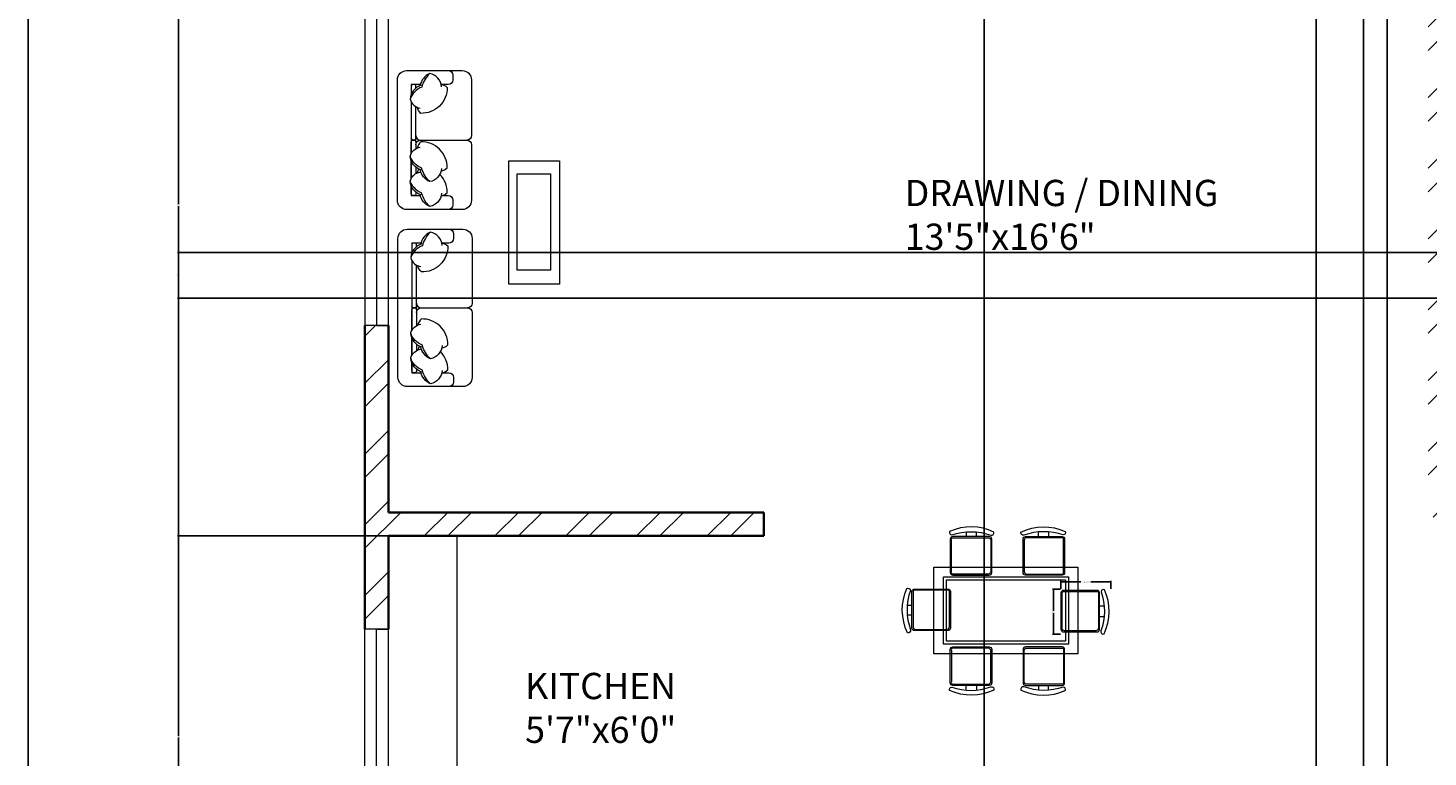
# Model space of a CAD drawing. Units: inches. Extents: x 2064 to 2782, y 1196 to 2299.
# Tile 5 of 11: x 2064 to 2331, y 1963 to 2102. Entities that reach past the tile are written whole.
import ezdxf

# ---------------------------------------------------------------- set-up
doc = ezdxf.new("R2010")
doc.units = ezdxf.units.IN
for name, color, linetype, lineweight in [('A-ANNO-DIMS', 2, 'Continuous', 18), ('A-ANNO-TTLB', 7, 'Continuous', 25), ('A-AREA-IDEN', 7, 'Continuous', 18), ('A-FLOR-CASE', 8, 'Continuous', 18), ('A-FURN', 8, 'Continuous', 13), ('A-GLAZ', 151, 'Continuous', 18), ('A-WALL', 7, 'Continuous', 35), ('A-WALL-PATT', 9, 'Continuous', 13)]:
    doc.layers.add(name, color=color, linetype=linetype, lineweight=lineweight)
doc.styles.get("Standard").update_dxf_attribs({"font": 'arial.ttf'})
doc.dimstyles.get("Standard").update_dxf_attribs({"dimtxt": 0.18, "dimasz": 0.18, "dimexe": 0.18, "dimexo": 0.0625, "dimgap": 0.09, "dimtad": 0, "dimtih": 1, "dimtoh": 1, "dimdec": 4, "dimzin": 0, "dimdsep": 46, "dimtxsty": 'Standard', "dimcen": 0.09, "dimadec": 0, "dimazin": 0, "dimtfac": 1, "dimtdec": 4, "dimtofl": 0, "dimtmove": 0, "dimatfit": 3, "dimfxl": 1, "dimtolj": 1, "dimtzin": 0, "dimarcsym": 0})

# ---------------------------------------------------------------- blocks, each defined once
blk = doc.blocks.new('WIN-60IN')
for p, q in [((0, 4.5), (0, 0)), ((60, 4.5), (0, 4.5)), ((60, 2.25), (60, 4.5)), ((60, 4.5), (60, 0)), ((0, 0), (0, 2.25)), ((0, 2.25), (60, 2.25)), ((0, 0), (60, 0))]:
    blk.add_line(p, q)
blk = doc.blocks.new('WIN-36IN')
for p, q in [((0, 36), (4.5, 36)), ((0, 36), (0, 0)), ((4.5, 36), (2.25, 36)), ((2.25, 36), (2.25, 0)), ((4.5, 36), (4.5, 0)), ((2.25, 0), (0, 0)), ((0, 0), (4.5, 0))]:
    blk.add_line(p, q)
blk = doc.blocks.new('CHAIR-DINING')
for points in [[(7.35, 7.85, 0.414214), (6.87, 8.33), (0.49, 8.33, 0.414214), (0, 7.85), (0, 0.91, 0.414214), (0.49, 0.42), (6.87, 0.42, 0.414214), (7.35, 0.91), (7.35, 7.85)], [(7.35, 7.85, 0.414214), (6.87, 8.33), (0.49, 8.33, 0.414214), (0, 7.85), (0, 0.91, 0.414214), (0.49, 0.42), (6.87, 0.42, 0.414214), (7.35, 0.91), (7.35, 7.85)], [(7.65, 8.06, -0.175809), (7.6, 0.59, 0.578392), (8.22, 0.02, 0.214524), (8.33, 8.46, 0.552014), (7.65, 8.06, -0.065079)], [(7.65, 8.06, -0.175809), (7.6, 0.59, 0.578392), (8.22, 0.02, 0.214524), (8.33, 8.46, 0.552014), (7.65, 8.06, -0.065079)], [(7.35, 3.34), (8.23, 3.34, -0.064759)], [(7.35, 3.34), (8.23, 3.34, -0.064759)]]:
    blk.add_lwpolyline(points, format="xyb")
for points in [[(7.13, 7.84), (7.13, 1.13, -0.414214), (6.65, 0.64), (0.7, 0.64, -0.414214), (0.22, 1.13), (0.22, 7.84, -0.512069), (0.7, 8.11), (6.65, 8.11, -0.512069)], [(7.13, 7.84), (7.13, 1.12, -0.414214), (6.65, 0.64), (0.7, 0.64, -0.414214), (0.22, 1.12), (0.22, 7.84, -0.512069), (0.7, 8.11), (6.65, 8.11, -0.512069)]]:
    blk.add_lwpolyline(points, format="xyb", close=True)
blk.add_lwpolyline([(8.25, 5.29), (7.35, 5.29)])
blk.add_lwpolyline([(8.25, 5.29), (7.35, 5.29)])
blk = doc.blocks.new('TABLE-DINING')
for points in [[(0, 16.47), (27.45, 16.47), (27.45, 0), (0, 0)], [(0, 16.47), (27.45, 16.47), (27.45, 0), (0, 0)], [(1.83, 14.64), (25.62, 14.64), (25.62, 1.83), (1.83, 1.83)], [(1.83, 14.64), (25.62, 14.64), (25.62, 1.83), (1.83, 1.83)], [(2.38, 14.09), (25.07, 14.09), (25.07, 2.38), (2.38, 2.38)], [(2.38, 14.09), (25.07, 14.09), (25.07, 2.38), (2.38, 2.38)]]:
    blk.add_lwpolyline(points, close=True)
blk = doc.blocks.new('TABLE-COFFEE')
for points in [[(0, 23.5), (9.66, 23.5), (9.66, 0), (0, 0)], [(1.54, 21.03), (7.9, 21.03), (7.9, 2.7), (1.54, 2.7)]]:
    blk.add_lwpolyline(points, close=True)
blk = doc.blocks.new('*D18')
at = {"layer": 'A-ANNO-DIMS', "color": 0, "lineweight": -2, "transparency": 16777216}
for p, q in [((2260.79, 1994.7), (2260.79, 1996.25)), ((2260.97, 1996.07), (2264.58, 1996.07)), ((2270.11, 1996.07), (2266.49, 1996.07)), ((2270.29, 1994.7), (2270.29, 1996.25))]:
    blk.add_line(p, q, dxfattribs=at)
at = {"layer": 'A-ANNO-DIMS', "color": 0, "transparency": 16777216}
for points in [[(2260.97, 1996.1), (2260.97, 1996.04), (2260.79, 1996.07)], [(2270.11, 1996.1), (2270.11, 1996.04), (2270.29, 1996.07)]]:
    blk.add_solid(points, dxfattribs=at)
at = {"layer": 'Defpoints', "color": 0, "transparency": 16777216}
for p in [(2270.29, 1996.07), (2260.79, 1994.64), (2270.29, 1994.64)]:
    blk.add_point(p, dxfattribs=at)
at = {"layer": 'A-ANNO-DIMS', "color": 0, "transparency": 16777216, "insert": (2265.54, 1996.07), "char_height": 0.18, "attachment_point": 5}
blk.add_mtext('\\A1;CHAIR 10 TYP.', dxfattribs=at)
blk = doc.blocks.new('*D19')
at = {"layer": 'A-ANNO-DIMS', "color": 0, "lineweight": -2, "transparency": 16777216}
for p, q in [((2260.72, 1994.64), (2259.18, 1994.64)), ((2259.36, 1994.46), (2259.36, 1990.54)), ((2259.36, 1986.26), (2259.36, 1990.18)), ((2260.72, 1986.08), (2259.18, 1986.08))]:
    blk.add_line(p, q, dxfattribs=at)
at = {"layer": 'A-ANNO-DIMS', "color": 0, "transparency": 16777216}
for points in [[(2259.33, 1994.46), (2259.39, 1994.46), (2259.36, 1994.64)], [(2259.33, 1986.26), (2259.39, 1986.26), (2259.36, 1986.08)]]:
    blk.add_solid(points, dxfattribs=at)
at = {"layer": 'Defpoints', "color": 0, "transparency": 16777216}
for p in [(2259.36, 1994.64), (2260.79, 1994.64), (2260.79, 1986.08)]:
    blk.add_point(p, dxfattribs=at)
at = {"layer": 'A-ANNO-DIMS', "color": 0, "transparency": 16777216, "insert": (2259.36, 1990.36), "char_height": 0.18, "attachment_point": 5}
blk.add_mtext('\\A1;9 TYP.', dxfattribs=at)
blk = doc.blocks.new('*D26')
at = {"layer": 'A-ANNO-DIMS', "color": 0, "lineweight": -2, "transparency": 16777216}
for p, q in [((2246.18, 1643.35), (2246.18, 2269.97)), ((2246.36, 2269.79), (2281.92, 2269.79)), ((2318.27, 2269.79), (2282.71, 2269.79)), ((2318.45, 1640.85), (2318.45, 2269.97))]:
    blk.add_line(p, q, dxfattribs=at)
at = {"layer": 'A-ANNO-DIMS', "color": 0, "transparency": 16777216}
for points in [[(2246.36, 2269.82), (2246.36, 2269.76), (2246.18, 2269.79)], [(2318.27, 2269.82), (2318.27, 2269.76), (2318.45, 2269.79)]]:
    blk.add_solid(points, dxfattribs=at)
at = {"layer": 'Defpoints', "color": 0, "transparency": 16777216}
for p in [(2318.45, 2269.79), (2246.18, 1643.29), (2318.45, 1640.79)]:
    blk.add_point(p, dxfattribs=at)
at = {"layer": 'A-ANNO-DIMS', "color": 0, "transparency": 16777216, "insert": (2282.32, 2269.79), "char_height": 0.18, "attachment_point": 5}
blk.add_mtext('\\A1;72.27', dxfattribs=at)
blk = doc.blocks.new('*D31')
at = {"layer": 'A-ANNO-DIMS', "color": 0, "lineweight": -2, "transparency": 16777216}
for p, q in [((2132.61, 2004.79), (2092.49, 2004.79)), ((2092.67, 2004.61), (2092.67, 1966.72)), ((2092.67, 1928.47), (2092.67, 1966.36)), ((2132.61, 1928.29), (2092.49, 1928.29))]:
    blk.add_line(p, q, dxfattribs=at)
at = {"layer": 'A-ANNO-DIMS', "color": 0, "transparency": 16777216}
for points in [[(2092.64, 2004.61), (2092.7, 2004.61), (2092.67, 2004.79)], [(2092.64, 1928.47), (2092.7, 1928.47), (2092.67, 1928.29)]]:
    blk.add_solid(points, dxfattribs=at)
at = {"layer": 'Defpoints', "color": 0, "transparency": 16777216}
for p in [(2092.67, 2004.79), (2132.67, 2004.79), (2132.67, 1928.29)]:
    blk.add_point(p, dxfattribs=at)
at = {"layer": 'A-ANNO-DIMS', "color": 0, "transparency": 16777216, "insert": (2092.67, 1966.54), "char_height": 0.18, "attachment_point": 5}
blk.add_mtext('\\A1;76.5', dxfattribs=at)
blk = doc.blocks.new('*D32')
at = {"layer": 'A-ANNO-DIMS', "color": 0, "lineweight": -2, "transparency": 16777216}
for p, q in [((2132.61, 2130.79), (2092.49, 2130.79)), ((2092.67, 2130.61), (2092.67, 2067.97)), ((2092.67, 2004.97), (2092.67, 2067.61)), ((2132.61, 2004.79), (2092.49, 2004.79))]:
    blk.add_line(p, q, dxfattribs=at)
at = {"layer": 'A-ANNO-DIMS', "color": 0, "transparency": 16777216}
for points in [[(2092.64, 2130.61), (2092.7, 2130.61), (2092.67, 2130.79)], [(2092.64, 2004.97), (2092.7, 2004.97), (2092.67, 2004.79)]]:
    blk.add_solid(points, dxfattribs=at)
at = {"layer": 'Defpoints', "color": 0, "transparency": 16777216}
for p in [(2092.67, 2130.79), (2132.67, 2130.79), (2132.67, 2004.79)]:
    blk.add_point(p, dxfattribs=at)
at = {"layer": 'A-ANNO-DIMS', "color": 0, "transparency": 16777216, "insert": (2092.67, 2067.79), "char_height": 0.18, "attachment_point": 5}
blk.add_mtext('\\A1;126', dxfattribs=at)
blk = doc.blocks.new('*D35')
at = {"layer": 'A-ANNO-DIMS', "color": 0, "lineweight": -2, "transparency": 16777216}
for p, q in [((2309.4, 1932.85), (2309.4, 2269.97)), ((2309.58, 2269.79), (2347.37, 2269.79)), ((2385.94, 2269.79), (2348.16, 2269.79)), ((2386.12, 1856.35), (2386.12, 2269.97))]:
    blk.add_line(p, q, dxfattribs=at)
at = {"layer": 'A-ANNO-DIMS', "color": 0, "transparency": 16777216}
for points in [[(2309.58, 2269.82), (2309.58, 2269.76), (2309.4, 2269.79)], [(2385.94, 2269.82), (2385.94, 2269.76), (2386.12, 2269.79)]]:
    blk.add_solid(points, dxfattribs=at)
at = {"layer": 'Defpoints', "color": 0, "transparency": 16777216}
for p in [(2386.12, 2269.79), (2309.4, 1932.79), (2386.12, 1856.29)]:
    blk.add_point(p, dxfattribs=at)
at = {"layer": 'A-ANNO-DIMS', "color": 0, "transparency": 16777216, "insert": (2347.76, 2269.79), "char_height": 0.18, "attachment_point": 5}
blk.add_mtext('\\A1;76.72', dxfattribs=at)
blk = doc.blocks.new('*D39')
at = {"layer": 'A-ANNO-DIMS', "color": 0, "lineweight": -2, "transparency": 16777216}
for p, q in [((2322.95, 1645.35), (2322.95, 2269.97)), ((2323.13, 2269.79), (2333.59, 2269.79)), ((2344.97, 2269.79), (2334.51, 2269.79)), ((2345.15, 1645.35), (2345.15, 2269.97))]:
    blk.add_line(p, q, dxfattribs=at)
at = {"layer": 'A-ANNO-DIMS', "color": 0, "transparency": 16777216}
for points in [[(2323.13, 2269.82), (2323.13, 2269.76), (2322.95, 2269.79)], [(2344.97, 2269.82), (2344.97, 2269.76), (2345.15, 2269.79)]]:
    blk.add_solid(points, dxfattribs=at)
at = {"layer": 'Defpoints', "color": 0, "transparency": 16777216}
for p in [(2345.15, 2269.79), (2322.95, 1645.29), (2345.15, 1645.29)]:
    blk.add_point(p, dxfattribs=at)
at = {"layer": 'A-ANNO-DIMS', "color": 0, "transparency": 16777216, "insert": (2334.05, 2269.79), "char_height": 0.18, "attachment_point": 5}
blk.add_mtext('\\A1;22.194', dxfattribs=at)
blk = doc.blocks.new('*D40')
at = {"layer": 'A-ANNO-DIMS', "color": 0, "lineweight": -2, "transparency": 16777216}
for p, q in [((2648.61, 2058.79), (2092.49, 2058.79)), ((2092.67, 2058.61), (2092.67, 2054.63)), ((2092.67, 2050.29), (2092.67, 2054.27)), ((2648.61, 2050.11), (2092.49, 2050.11))]:
    blk.add_line(p, q, dxfattribs=at)
at = {"layer": 'A-ANNO-DIMS', "color": 0, "transparency": 16777216}
for points in [[(2092.64, 2058.61), (2092.7, 2058.61), (2092.67, 2058.79)], [(2092.64, 2050.29), (2092.7, 2050.29), (2092.67, 2050.11)]]:
    blk.add_solid(points, dxfattribs=at)
at = {"layer": 'Defpoints', "color": 0, "transparency": 16777216}
for p in [(2092.67, 2058.79), (2648.67, 2058.79), (2648.67, 2050.11)]:
    blk.add_point(p, dxfattribs=at)
at = {"layer": 'A-ANNO-DIMS', "color": 0, "transparency": 16777216, "insert": (2092.67, 2054.45), "char_height": 0.18, "attachment_point": 5}
blk.add_mtext('\\A1;8.682', dxfattribs=at)

msp = doc.modelspace()

# ---------------------------------------------------------------- hatches: boundary and pattern name
at = {"layer": 'A-WALL-PATT'}
h = msp.add_hatch(dxfattribs=at)
h.set_pattern_fill('ANSI32', color=256)
h.paths.add_polyline_path([(2489.7688, 2189.2917), (2574.5454, 2189.2917), (2574.5454, 2191.5417), (2574.5454, 2193.7917), (2570.6691, 2193.7917), (2570.6691, 2197.3052), (2568.4191, 2197.3052), (2566.1691, 2197.3052), (2566.1691, 2193.7917), (2494.1691, 2193.7917), (2494.1691, 2229.7917), (2523.2441, 2229.7917), (2523.2441, 2234.2917), (2471.2886, 2234.2917), (2471.2886, 2229.7917), (2489.6691, 2229.7917), (2489.6691, 2193.7917), (2417.6691, 2193.7917), (2417.6691, 2197.0632), (2415.4191, 2197.0632), (2413.1691, 2197.0632), (2413.1691, 2193.7917), (2406.8865, 2193.7917), (2406.8865, 2189.2917), (2485.2688, 2189.2917), (2485.2688, 2063.2917), (2369.1629, 2063.2917), (2369.1629, 2058.7917), (2386.1222, 2058.7917), (2386.1222, 1856.2917), (2382.1576, 1856.2917), (2382.1576, 1851.7917), (2394.9764, 1851.7917), (2394.9764, 1854.0417), (2394.9764, 1856.2917), (2390.6222, 1856.2917), (2390.6222, 2058.7917), (2485.2688, 2058.7917), (2493.762, 2058.7917), (2493.762, 2061.0417), (2493.762, 2063.2917), (2489.7688, 2063.2917)])
h.paths.add_polyline_path([(2447.2886, 2234.2917), (2413.1691, 2234.2917), (2413.1691, 2217.3799), (2417.6691, 2217.3799), (2417.6691, 2229.7917), (2447.2886, 2229.7917)], flags=17)
h.paths.add_polyline_path([(2570.6691, 2234.2917), (2547.2441, 2234.2917), (2547.2441, 2229.7917), (2566.1691, 2229.7917), (2566.1691, 2216.5615), (2570.6691, 2216.5615)], flags=17)
h.paths.add_polyline_path([(2653.1691, 2189.2917), (2653.1691, 2193.7917), (2640.8843, 2193.7917), (2640.8843, 2189.2917), (2648.6691, 2189.2917), (2648.6691, 2162.7138), (2653.1691, 2162.7138)])
h.paths.add_polyline_path([(2653.1691, 2102.7138), (2648.6691, 2102.7138), (2648.6691, 2063.2917), (2526.7281, 2063.2917), (2526.7281, 2058.7917), (2541.1691, 2058.7917), (2541.1691, 1993.2917), (2545.6691, 1993.2917), (2545.6691, 1997.7917), (2545.6691, 2058.7917), (2648.6691, 2058.7917), (2648.6691, 2050.1099), (2653.1691, 2050.1099)])
h.paths.add_polyline_path([(2600.6691, 1856.2917), (2493.4607, 1856.2917), (2493.4607, 1851.7917), (2596.1691, 1851.7917), (2596.1691, 1695.7917), (2594.0816, 1695.7917), (2594.0816, 1691.2917), (2614.7905, 1691.2917), (2614.7905, 1645.2917), (2536.7905, 1645.2917), (2536.7905, 1691.2917), (2539.332, 1691.2917), (2539.332, 1693.5417), (2539.332, 1695.7917), (2452.1691, 1695.7917), (2452.1691, 1851.7917), (2456.0775, 1851.7917), (2456.0775, 1856.2917), (2427.1536, 1856.2917), (2427.1536, 1851.7917), (2447.6691, 1851.7917), (2447.6691, 1695.7917), (2447.6691, 1645.2917), (2405.1469, 1645.2917), (2405.1469, 1640.7917), (2452.1691, 1640.7917), (2452.1691, 1645.2917), (2452.1691, 1691.2917), (2534.7905, 1691.2917), (2534.7905, 1645.2917), (2534.7905, 1643.2917), (2614.7905, 1643.2917), (2616.7905, 1643.2917), (2616.7905, 1691.2917), (2622.4029, 1691.2917), (2622.4029, 1693.7143), (2622.4029, 1695.7917), (2600.6691, 1695.7917), (2600.6691, 1779.7917), (2648.6691, 1779.7917), (2648.6691, 1695.7917), (2646.4029, 1695.7917), (2646.4029, 1691.2917), (2653.1691, 1691.2917), (2653.1691, 1906.3508), (2648.6691, 1906.3508), (2648.6691, 1856.2917), (2648.6691, 1784.2917), (2600.6691, 1784.2917)])
h.paths.add_polyline_path([(2322.9532, 1819.5181), (2320.7032, 1819.5181), (2318.4532, 1819.5181), (2318.4532, 1695.7917), (2242.7664, 1695.7917), (2242.7664, 1691.2917), (2318.4532, 1691.2917), (2318.4532, 1640.7917), (2322.9532, 1640.7917), (2345.1469, 1640.7917), (2345.1469, 1643.0417), (2345.1469, 1645.2917), (2322.9532, 1645.2917), (2322.9532, 1691.2917), (2322.9532, 1695.7917)])
h.paths.add_polyline_path([(2166.1825, 1691.2917), (2164.1825, 1691.2917), (2164.1825, 1643.2917), (2166.1825, 1643.2917), (2246.1825, 1643.2917), (2246.1825, 1645.2917), (2246.1825, 1691.2917), (2244.1825, 1691.2917), (2244.1825, 1645.2917), (2166.1825, 1645.2917)])
h.paths.add_polyline_path([(2309.404, 1932.7917), (2204.1691, 1932.7917), (2204.1691, 1960.0962), (2199.6691, 1960.0962), (2199.6691, 1932.7917), (2132.6691, 1932.7917), (2132.6691, 1951.0737), (2128.1691, 1951.0737), (2128.1691, 1910.0412), (2132.6691, 1910.0412), (2132.6691, 1928.2917), (2304.904, 1928.2917), (2304.904, 1856.2917), (2304.904, 1851.7917), (2318.4532, 1851.7917), (2318.4532, 1848.8308), (2322.9532, 1848.8308), (2322.9532, 1851.7917), (2347.7631, 1851.7917), (2347.7631, 1856.2917), (2309.404, 1856.2917)])
h.paths.add_polyline_path([(2132.6691, 2044.9092), (2130.4191, 2044.9092), (2128.1691, 2044.9092), (2128.1691, 1987.0737), (2132.6691, 1987.0737), (2132.6691, 2004.7917), (2199.6691, 2004.7917), (2204.1691, 2004.7917), (2204.1691, 2009.2917), (2132.6691, 2009.2917)])
h.paths.add_polyline_path([(2186.6691, 2195.9329), (2184.4191, 2195.9329), (2184.4191, 2195.8929), (2182.1691, 2195.9329), (2182.1691, 2193.7917), (2128.1691, 2193.7917), (2128.1691, 2181.4967), (2132.6691, 2181.4967), (2132.6691, 2182.7769), (2132.6691, 2189.2917), (2182.1691, 2189.2917), (2182.1691, 2135.2917), (2179.804, 2135.2917), (2179.804, 2130.7917), (2190.215, 2130.7917), (2190.215, 2133.0417), (2190.215, 2135.2917), (2186.6691, 2135.2917)])
h.paths.add_polyline_path([(2340.0628, 2189.2917), (2340.0628, 2191.5417), (2340.0628, 2193.7917), (2335.1691, 2193.7917), (2335.1691, 2234.2917), (2280.6746, 2234.2917), (2280.6746, 2229.7917), (2330.6691, 2229.7917), (2330.6691, 2193.7917), (2330.6691, 2135.2917), (2218.6309, 2135.2917), (2218.6309, 2130.7917), (2330.7688, 2130.7917), (2330.7688, 2008.4023), (2335.2688, 2008.4023), (2335.2688, 2058.7917), (2338.9208, 2058.7917), (2338.9208, 2061.0417), (2338.9208, 2063.2917), (2335.2688, 2063.2917), (2335.2688, 2189.2917)])
h.paths.add_polyline_path([(2220.6746, 2234.2917), (2182.1691, 2234.2917), (2182.1691, 2227.4187), (2186.6691, 2227.4187), (2186.6691, 2229.7917), (2220.6746, 2229.7917), (2220.6746, 2232.0417)])
h.paths.add_polyline_path([(2158.8146, 2135.2917), (2132.6691, 2135.2917), (2132.6691, 2157.4967), (2128.1691, 2157.4967), (2128.1691, 2104.9092), (2132.6691, 2104.9092), (2132.6691, 2130.7917), (2158.8146, 2130.7917), (2158.8146, 2133.0417)])
h.paths.add_polyline_path([(2396.0464, 2062.2045), (2434.8868, 2062.2045), (2434.8868, 2080.8619), (2396.0464, 2080.8619)], flags=24)
h.paths.add_polyline_path([(2196.1396, 1653.3449), (2232.023, 1653.3449), (2232.023, 1672.0022), (2196.1396, 1672.0022)], flags=25)

# ---------------------------------------------------------------- linework, layer by layer
at = {"layer": 'A-ANNO-TTLB'}
msp.add_lwpolyline([(2063.9994, 2298.574), (2782.0941, 2298.574), (2782.0941, 1490.6238), (2063.9994, 1490.6238)], close=True, dxfattribs=at)
at = {"layer": 'A-FLOR-CASE'}
msp.add_line((2145.6809, 2004.7917), (2145.6809, 1946.3811), dxfattribs=at)
at = {"layer": 'A-FURN', "ltscale": 0.03}
for points in [[(2148.4815, 2081.0868, -0.41421356), (2147.5995, 2080.2048, -0.41421356), (2148.4815, 2079.3228), (2148.4815, 2068.7388, -0.41421356), (2146.7175, 2066.9749), (2136.1335, 2066.9749, -0.41421356), (2134.3695, 2068.7388), (2134.3695, 2091.6708, -0.41421356), (2136.1335, 2093.4348), (2146.7175, 2093.4348, -0.41421356), (2148.4815, 2091.6708), (2148.4815, 2081.0868, -0.41421356), (2147.5995, 2080.2048, -0.41421356), (2148.4815, 2079.3228)], [(2148.6, 2049.114, -0.41421356), (2147.718, 2048.232, -0.41421356), (2148.6, 2047.35), (2148.6, 2035.002, -0.41421356), (2146.836, 2033.238), (2136.252, 2033.238, -0.41421356), (2134.488, 2035.002), (2134.488, 2061.4619, -0.41421356), (2136.252, 2063.2259), (2146.836, 2063.2259, -0.41421356), (2148.6, 2061.4619), (2148.6, 2049.114, -0.41421356), (2147.718, 2048.232, -0.41421356), (2148.6, 2047.35)]]:
    msp.add_lwpolyline(points, format="xyb", dxfattribs=at)
at = {"layer": 'A-FURN'}
for points in [[(2140.5352, 2092.8734, 0.14772988), (2139.0194, 2090.2956, 0.21334276), (2136.7962, 2088.0211, 0.17866181)], [(2142.7584, 2090.3462, 0.35677236), (2140.5352, 2092.8734, 0.24954205), (2138.7031, 2090.5835, -9.61688035)], [(2144.0715, 2093.4348, -0.41421356), (2144.9535, 2092.5528), (2144.9535, 2091.6708, -0.41421356), (2144.0715, 2090.7888), (2142.705, 2090.7888)], [(2138.8986, 2090.6517, 0.30666349), (2136.7962, 2088.0211, 0.30632997), (2138.7162, 2086.3025, -0.87284716)], [(2137.8975, 2090.1157), (2137.8975, 2090.436, 0.41421356), (2137.5447, 2090.7888), (2137.3683, 2090.7888, 0.41421356), (2137.0155, 2090.436)], [(2137.0155, 2090.436), (2137.0155, 2088.9333, 0.41421356)], [(2142.7046, 2090.7907, -0.16554063), (2143.8699, 2090.2451, -0.42598917), (2138.8173, 2085.2916, -0.12152332), (2138.1209, 2086.4675, 7.11546429)], [(2137.0155, 2087.466), (2137.0155, 2080.5576, 0.41421356), (2137.3683, 2080.2048), (2137.5447, 2080.2048, 0.41421356), (2137.8975, 2080.5576), (2137.8975, 2086.5779, 0.41421356)], [(2137.8975, 2081.0868, 0.41421356), (2138.7795, 2080.2048)], [(2137.8975, 2081.0868, 0.41421356), (2138.7795, 2080.2048), (2147.5995, 2080.2048, 0.41421356)], [(2138.8986, 2074.5092, -0.30666349), (2136.7962, 2077.1398, -0.30632997), (2138.7162, 2078.8584, 0.87284716)], [(2137.0155, 2077.6949), (2137.0155, 2079.852, -0.41421356), (2137.3683, 2080.2048), (2137.5447, 2080.2048, -0.41421356), (2137.8975, 2079.852), (2137.8975, 2078.583, -0.41421356)], [(2137.8975, 2079.3228, -0.41421356), (2138.7795, 2080.2048)], [(2137.8975, 2079.3228, -0.41421356), (2138.7795, 2080.2048), (2147.5995, 2080.2048, -0.41421356)], [(2142.7046, 2074.3702, 0.16554063), (2143.8699, 2074.9158, 0.42598917), (2138.8173, 2079.8693, 0.12152332), (2138.1209, 2078.6935, -7.11546429)], [(2140.5352, 2072.2875, -0.14772988), (2139.0194, 2074.8653, -0.21334276), (2136.7962, 2077.1398, -0.17866181)], [(2137.0155, 2072.9436), (2137.0155, 2076.2276, -0.41421356)], [(2138.8986, 2069.7579, -0.30666349), (2136.7962, 2072.3886, -0.30632997), (2138.7162, 2074.1071, 0.87284716)], [(2137.8975, 2075.0452), (2137.8975, 2073.8318, -0.41421356)], [(2138.4657, 2074.6816, 0.07186538), (2138.1209, 2073.9422, -7.11546429)], [(2142.7584, 2074.8148, -0.35677236), (2140.5352, 2072.2875, -0.24954205), (2138.7031, 2074.5774, 9.61688035)], [(2142.7046, 2069.6189, 0.16554063), (2143.8699, 2070.1646, 0.20023115), (2142.4506, 2073.6658, 0.12152332)], [(2140.5352, 2067.5362, -0.14772988), (2139.0194, 2070.114, -0.21334276), (2136.7962, 2072.3886, -0.17866181)], [(2137.0155, 2069.9736), (2137.0155, 2071.4763, -0.41421356)], [(2137.0155, 2071.4763), (2137.0155, 2069.6208), (2138.7489, 2069.6208, -0.41421356)], [(2137.8975, 2070.2939), (2137.8975, 2069.9736, -0.41421356), (2137.5447, 2069.6208), (2137.3683, 2069.6208, -0.41421356), (2137.0155, 2069.9736)], [(2142.7584, 2070.0635, -0.35677236), (2140.5352, 2067.5362, -0.24954205), (2138.7031, 2069.8261, 9.61688035)], [(2142.705, 2069.6208), (2144.0715, 2069.6208, -0.41421356), (2144.9535, 2068.7388), (2144.9535, 2067.8569, -0.41421356), (2144.0715, 2066.9749)], [(2140.6537, 2062.6646, 0.14772988), (2139.1379, 2060.0868, 0.21334276), (2136.9147, 2057.8122, 0.17866181)], [(2142.8769, 2060.1373, 0.35677236), (2140.6537, 2062.6646, 0.24954205), (2138.8216, 2060.3746, -9.61688035)], [(2144.19, 2063.2259, -0.41421356), (2145.072, 2062.3439), (2145.072, 2061.4619, -0.41421356), (2144.19, 2060.5799), (2142.8235, 2060.5799)], [(2139.0171, 2060.4429, 0.30666349), (2136.9147, 2057.8122, 0.30632997), (2138.8347, 2056.0937, -0.87284716)], [(2138.016, 2059.9069), (2138.016, 2060.2271, 0.41421356), (2137.6632, 2060.5799), (2137.4868, 2060.5799, 0.41421356), (2137.134, 2060.2271)], [(2137.134, 2060.2271), (2137.134, 2058.7244, 0.41421356)], [(2142.8231, 2060.5818, -0.16554063), (2143.9884, 2060.0362, -0.42598917), (2138.9358, 2055.0827, -0.12152332), (2138.2393, 2056.2586, 7.11546429)], [(2137.134, 2057.2571), (2137.134, 2048.5848, 0.41421356), (2137.4868, 2048.232), (2137.6632, 2048.232, 0.41421356), (2138.016, 2048.5848), (2138.016, 2056.369, 0.41421356)], [(2138.016, 2049.114, 0.41421356), (2138.898, 2048.232)], [(2138.016, 2049.114, 0.41421356), (2138.898, 2048.232), (2147.718, 2048.232, 0.41421356)], [(2137.134, 2043.9581), (2137.134, 2047.8792, -0.41421356), (2137.4868, 2048.232), (2137.6632, 2048.232, -0.41421356), (2138.016, 2047.8792), (2138.016, 2044.8462, -0.41421356)], [(2138.016, 2047.35, -0.41421356), (2138.898, 2048.232)], [(2138.016, 2047.35, -0.41421356), (2138.898, 2048.232), (2147.718, 2048.232, -0.41421356)], [(2142.8231, 2040.6334, 0.16554063), (2143.9884, 2041.179, 0.42598917), (2138.9358, 2046.1325, 0.12152332), (2138.2393, 2044.9566, -7.11546429)], [(2139.0171, 2040.7723, -0.30666349), (2136.9147, 2043.403, -0.30632997), (2138.8347, 2045.1216, 0.87284716)], [(2140.6537, 2038.5506, -0.14772988), (2139.1379, 2041.1285, -0.21334276), (2136.9147, 2043.403, -0.17866181)], [(2137.134, 2039.2068), (2137.134, 2042.4908, -0.41421356)], [(2138.016, 2041.3084), (2138.016, 2040.0949, -0.41421356)], [(2138.5842, 2040.9448, 0.07186538), (2138.2393, 2040.2053, -7.11546429)], [(2142.8769, 2041.0779, -0.35677236), (2140.6537, 2038.5506, -0.24954205), (2138.8216, 2040.8406, 9.61688035)], [(2139.0171, 2036.021, -0.30666349), (2136.9147, 2038.6517, -0.30632997), (2138.8347, 2040.3703, 0.87284716)], [(2140.6537, 2033.7993, -0.14772988), (2139.1379, 2036.3772, -0.21334276), (2136.9147, 2038.6517, -0.17866181)], [(2137.134, 2037.7395), (2137.134, 2035.884), (2138.8674, 2035.884, -0.41421356)], [(2137.134, 2036.2368), (2137.134, 2037.7395, -0.41421356)], [(2142.8231, 2035.8821, 0.16554063), (2143.9884, 2036.4277, 0.20023115), (2142.5691, 2039.9289, 0.12152332)], [(2138.016, 2036.5571), (2138.016, 2036.2368, -0.41421356), (2137.6632, 2035.884), (2137.4868, 2035.884, -0.41421356), (2137.134, 2036.2368)], [(2142.8769, 2036.3266, -0.35677236), (2140.6537, 2033.7993, -0.24954205), (2138.8216, 2036.0893, 9.61688035)], [(2142.8235, 2035.884), (2144.19, 2035.884, -0.41421356), (2145.072, 2035.002), (2145.072, 2034.12, -0.41421356), (2144.19, 2033.238)], [(2239.9772, 2004.9849, -0.17580919), (2247.4526, 2004.9283, 0.57839206), (2248.019, 2005.551, 0.21452438), (2239.5808, 2005.6643, 0.55201397), (2239.9772, 2004.9849, -0.06507904)], [(2239.9772, 2004.9846, -0.17580919), (2247.4527, 2004.928, 0.57839206), (2248.019, 2005.5508, 0.21452438), (2239.5808, 2005.664, 0.55201397), (2239.9772, 2004.9846, -0.06507904)], [(2253.746, 2004.9283, -0.57839206), (2253.1797, 2005.551, -0.21452438), (2261.6179, 2005.6643, -0.55201397), (2261.2214, 2004.9849, 0.1758092), (2253.746, 2004.9283)], [(2253.746, 2004.928, -0.57839206), (2253.1797, 2005.5508, -0.21452438), (2261.6179, 2005.664, -0.55201397), (2261.2214, 2004.9846, 0.1758092), (2253.746, 2004.928)], [(2247.1355, 2004.6849), (2240.1955, 2004.6849, 0.41421356), (2239.71, 2004.1994), (2239.71, 1997.8182, 0.41421356), (2240.1955, 1997.3327), (2247.1355, 1997.3327, 0.41421356), (2247.621, 1997.8182), (2247.621, 2004.1994, 0.41421356), (2247.1355, 2004.6849)], [(2247.1355, 2004.6846), (2240.1956, 2004.6846, 0.41421356), (2239.71, 2004.1991), (2239.71, 1997.8179, 0.41421356), (2240.1956, 1997.3324), (2247.1355, 1997.3324, 0.41421356), (2247.621, 1997.8179), (2247.621, 2004.1991, 0.41421356), (2247.1355, 2004.6846)], [(2244.6978, 2004.6849), (2244.6978, 2005.5626, -0.06475861)], [(2244.6978, 2004.6846), (2244.6978, 2005.5623, -0.06475861)], [(2261.0031, 2004.6849, -0.41421356), (2261.4886, 2004.1994), (2261.4886, 1997.8182, -0.41421356), (2261.0031, 1997.3327), (2254.0631, 1997.3327, -0.41421356), (2253.5776, 1997.8182), (2253.5776, 2004.1994, -0.41421356), (2254.0631, 2004.6849), (2261.0031, 2004.6849)], [(2261.0031, 2004.6846, -0.41421356), (2261.4886, 2004.1991), (2261.4886, 1997.8179, -0.41421356), (2261.0031, 1997.3324), (2254.0632, 1997.3324, -0.41421356), (2253.5776, 1997.8179), (2253.5776, 2004.1991, -0.41421356), (2254.0632, 2004.6846), (2261.0031, 2004.6846)], [(2256.5008, 2004.6849), (2256.5008, 2005.5626, 0.06475861)], [(2256.5008, 2004.6846), (2256.5008, 2005.5623, 0.06475861)], [(2232.1565, 1986.9329, -0.57839206), (2231.5337, 1986.3666, -0.21452438), (2231.4205, 1994.8048, -0.55201397), (2232.0998, 1994.4083, 0.17580937), (2232.1565, 1986.9329)], [(2232.1565, 1986.9326, -0.57839206), (2231.5338, 1986.3663, -0.21452438), (2231.4205, 1994.8045, -0.55201397), (2232.0999, 1994.408, 0.17580937), (2232.1565, 1986.9326)], [(2232.3999, 1994.19, -0.41421356), (2232.8854, 1994.6755), (2239.2665, 1994.6755, -0.41421356), (2239.7521, 1994.19), (2239.7521, 1987.25, -0.41421356), (2239.2665, 1986.7645), (2232.8854, 1986.7645, -0.41421356), (2232.3999, 1987.25), (2232.3999, 1994.19)], [(2232.3999, 1994.1897, -0.41421356), (2232.8854, 1994.6752), (2239.2666, 1994.6752, -0.41421356), (2239.7521, 1994.1897), (2239.7521, 1987.2498, -0.41421356), (2239.2666, 1986.7642), (2232.8854, 1986.7642, -0.41421356), (2232.3999, 1987.2498), (2232.3999, 1994.1897)], [(2232.3999, 1989.6877), (2231.5222, 1989.6877, 0.06475861)], [(2232.3999, 1989.6874), (2231.5222, 1989.6874, 0.06475861)], [(2247.1355, 1976.3192), (2240.1955, 1976.3192, -0.41421356), (2239.71, 1976.8047), (2239.71, 1983.1858, -0.41421356), (2240.1955, 1983.6714), (2247.1355, 1983.6714, -0.41421356), (2247.621, 1983.1858), (2247.621, 1976.8047, -0.41421356), (2247.1355, 1976.3192)], [(2247.1355, 1976.3189), (2240.1956, 1976.3189, -0.41421356), (2239.71, 1976.8044), (2239.71, 1983.1855, -0.41421356), (2240.1956, 1983.6711), (2247.1355, 1983.6711, -0.41421356), (2247.621, 1983.1855), (2247.621, 1976.8044, -0.41421356), (2247.1355, 1976.3189)], [(2261.0031, 1976.3192, 0.41421356), (2261.4886, 1976.8047), (2261.4886, 1983.1858, 0.41421356), (2261.0031, 1983.6714), (2254.0631, 1983.6714, 0.41421356), (2253.5776, 1983.1858), (2253.5776, 1976.8047, 0.41421356), (2254.0631, 1976.3192), (2261.0031, 1976.3192)], [(2261.0031, 1976.3189, 0.41421356), (2261.4886, 1976.8044), (2261.4886, 1983.1855, 0.41421356), (2261.0031, 1983.6711), (2254.0632, 1983.6711, 0.41421356), (2253.5776, 1983.1855), (2253.5776, 1976.8044, 0.41421356), (2254.0632, 1976.3189), (2261.0031, 1976.3189)], [(2247.4526, 1976.0757, -0.57839206), (2248.019, 1975.453, -0.21452438), (2239.5808, 1975.3398, -0.55201397), (2239.9772, 1976.0191, 0.17580929), (2247.4526, 1976.0757)], [(2247.4527, 1976.0754, -0.57839206), (2248.019, 1975.4527, -0.21452438), (2239.5808, 1975.3395, -0.55201397), (2239.9772, 1976.0188, 0.17580929), (2247.4527, 1976.0754)], [(2244.6978, 1976.3192), (2244.6978, 1975.4415, 0.06475861)], [(2244.6978, 1976.3189), (2244.6978, 1975.4412, 0.06475861)], [(2261.2214, 1976.0191, -0.17580928), (2253.746, 1976.0757, 0.57839206), (2253.1797, 1975.453, 0.21452438), (2261.6179, 1975.3398, 0.55201397), (2261.2214, 1976.0191, -0.06507904)], [(2261.2214, 1976.0188, -0.17580928), (2253.746, 1976.0754, 0.57839206), (2253.1797, 1975.4527, 0.21452438), (2261.6179, 1975.3395, 0.55201397), (2261.2214, 1976.0188, -0.06507904)], [(2256.5008, 1976.3192), (2256.5008, 1975.4415, -0.06475861)], [(2256.5008, 1976.3189), (2256.5008, 1975.4412, -0.06475861)]]:
    msp.add_lwpolyline(points, format="xyb", dxfattribs=at)
for points in [[(2138.7489, 2090.7888), (2137.0155, 2090.7888), (2137.0155, 2088.9333)], [(2137.0155, 2087.466), (2137.0155, 2077.6949)], [(2137.0155, 2076.2276), (2137.0155, 2072.9436)], [(2138.8674, 2060.5799), (2137.134, 2060.5799), (2137.134, 2058.7244)], [(2137.134, 2057.2571), (2137.134, 2043.9581)], [(2137.134, 2042.4908), (2137.134, 2039.2068)], [(2242.7552, 2005.5785), (2242.7552, 2004.6849)], [(2242.7553, 2005.5783), (2242.7553, 2004.6846)], [(2258.4434, 2005.5785), (2258.4434, 2004.6849)], [(2258.4434, 2005.5783), (2258.4434, 2004.6846)], [(2231.5062, 1991.6303), (2232.3999, 1991.6303)], [(2231.5063, 1991.63), (2232.3999, 1991.63)], [(2242.7552, 1975.4255), (2242.7552, 1976.3192)], [(2242.7553, 1975.4252), (2242.7553, 1976.3189)], [(2258.4434, 1975.4255), (2258.4434, 1976.3192)], [(2258.4434, 1975.4252), (2258.4434, 1976.3189)]]:
    msp.add_lwpolyline(points, dxfattribs=at)
for points in [[(2137.0155, 2080.5576), (2137.0155, 2079.852, -0.41421356), (2137.3683, 2080.2048), (2137.5447, 2080.2048, -0.41421356), (2137.8975, 2079.852), (2137.8975, 2080.5576, -0.41421356), (2137.5447, 2080.2048), (2137.3683, 2080.2048, -0.41421356)], [(2137.134, 2048.5848), (2137.134, 2047.8792, -0.41421356), (2137.4868, 2048.232), (2137.6632, 2048.232, -0.41421356), (2138.016, 2047.8792), (2138.016, 2048.5848, -0.41421356), (2137.6632, 2048.232), (2137.4868, 2048.232, -0.41421356)], [(2240.1985, 2004.4662), (2246.9168, 2004.4662, -0.41421356), (2247.4023, 2003.9806), (2247.4023, 1998.037, -0.41421356), (2246.9168, 1997.5514), (2240.1985, 1997.5514, -0.51206948), (2239.9288, 1998.037), (2239.9288, 2003.9806, -0.51206948)], [(2240.1985, 2004.4659), (2246.9168, 2004.4659, -0.41421356), (2247.4023, 2003.9804), (2247.4023, 1998.0367, -0.41421356), (2246.9168, 1997.5512), (2240.1985, 1997.5512, -0.51206948), (2239.9288, 1998.0367), (2239.9288, 2003.9804, -0.51206948)], [(2261.0001, 2004.4662), (2254.2819, 2004.4662, 0.41421356), (2253.7963, 2003.9806), (2253.7963, 1998.037, 0.41421356), (2254.2819, 1997.5514), (2261.0001, 1997.5514, 0.51206948), (2261.2699, 1998.037), (2261.2699, 2003.9806, 0.51206948)], [(2261.0002, 2004.4659), (2254.2819, 2004.4659, 0.41421356), (2253.7964, 2003.9804), (2253.7964, 1998.0367, 0.41421356), (2254.2819, 1997.5512), (2261.0002, 1997.5512, 0.51206948), (2261.2699, 1998.0367), (2261.2699, 2003.9804, 0.51206948)], [(2232.6186, 1994.187), (2232.6186, 1987.4688, 0.41421356), (2233.1041, 1986.9832), (2239.0478, 1986.9832, 0.41421356), (2239.5333, 1987.4688), (2239.5333, 1994.187, 0.51206948), (2239.0478, 1994.4568), (2233.1041, 1994.4568, 0.51206948)], [(2232.6186, 1994.1867), (2232.6186, 1987.4685, 0.41421356), (2233.1042, 1986.983), (2239.0478, 1986.983, 0.41421356), (2239.5334, 1987.4685), (2239.5334, 1994.1867, 0.51206948), (2239.0478, 1994.4565), (2233.1042, 1994.4565, 0.51206948)], [(2240.1985, 1976.5379), (2246.9168, 1976.5379, 0.41421356), (2247.4023, 1977.0234), (2247.4023, 1982.9671, 0.41421356), (2246.9168, 1983.4526), (2240.1985, 1983.4526, 0.51206948), (2239.9288, 1982.9671), (2239.9288, 1977.0234, 0.51206948)], [(2240.1985, 1976.5376), (2246.9168, 1976.5376, 0.41421356), (2247.4023, 1977.0231), (2247.4023, 1982.9668, 0.41421356), (2246.9168, 1983.4523), (2240.1985, 1983.4523, 0.51206948), (2239.9288, 1982.9668), (2239.9288, 1977.0231, 0.51206948)], [(2261.0001, 1976.5379), (2254.2819, 1976.5379, -0.41421356), (2253.7963, 1977.0234), (2253.7963, 1982.9671, -0.41421356), (2254.2819, 1983.4526), (2261.0001, 1983.4526, -0.51206948), (2261.2699, 1982.9671), (2261.2699, 1977.0234, -0.51206948)], [(2261.0002, 1976.5376), (2254.2819, 1976.5376, -0.41421356), (2253.7964, 1977.0231), (2253.7964, 1982.9668, -0.41421356), (2254.2819, 1983.4523), (2261.0002, 1983.4523, -0.51206948), (2261.2699, 1982.9668), (2261.2699, 1977.0231, -0.51206948)]]:
    msp.add_lwpolyline(points, format="xyb", close=True, dxfattribs=at)
at = {"layer": 'A-WALL'}
for p, q in [((2128.1691, 2044.9092), (2128.1691, 1987.0737)), ((2132.6691, 2044.9092), (2132.6691, 2009.2917)), ((2132.6691, 2009.2917), (2204.1691, 2009.2917)), ((2204.1691, 2009.2917), (2204.1691, 2004.7917)), ((2132.6691, 2004.7917), (2199.6691, 2004.7917)), ((2132.6691, 2004.7917), (2132.6691, 1987.0737)), ((2199.6691, 2004.7917), (2204.1691, 2004.7917))]:
    msp.add_line(p, q, dxfattribs=at)

# ---------------------------------------------------------------- block references
at = {"layer": 'A-FURN'}
for name, p in [('TABLE-COFFEE', (2155.6215, 2052.7508)), ('TABLE-DINING', (2236.5824, 1982.3562)), ('CHAIR-DINING', (2260.7851, 1986.1059))]:
    msp.add_blockref(name, p, dxfattribs=at)
at = {"layer": 'A-GLAZ'}
for name, p, rotation in [('WIN-60IN', (2128.1691, 2104.9092), 270), ('WIN-36IN', (2132.6691, 1987.0737), 180)]:
    msp.add_blockref(name, p, dxfattribs=dict(at, rotation=rotation))

# ---------------------------------------------------------------- texts
at = {"layer": 'A-AREA-IDEN', "char_height": 5, "attachment_point": 1}
for s, width, insert in [('DRAWING / DINING\\P13\'5"x16\'6"', 232.714386, (2231.0235, 2072.6283)), ('KITCHEN\\P5\'7"x6\'0"', 136.324724, (2158.7123, 1978.718))]:
    msp.add_mtext_dynamic_manual_height_columns(s, width=width, gutter_width=12.5, heights=[0], dxfattribs=dict(at, insert=insert))

# ---------------------------------------------------------------- dimensions: what is measured, and where the dimension line sits
at = {"layer": 'A-ANNO-DIMS'}
for base, p1, p2, override, picture, middle in [((2318.4532, 2269.7917), (2246.1825, 1643.2917), (2318.4532, 1640.7917), {"dimdec": 2, "dimlfac": 1, "dimrnd": 0, "dimzin": 0, "dimdsep": 46, "dimlunit": 2}, '*D26', (2282.3178, 2269.7917)), ((2386.1222, 2269.7917), (2309.404, 1932.7917), (2386.1222, 1856.2917), {"dimdec": 2, "dimlfac": 1, "dimrnd": 0, "dimzin": 0, "dimdsep": 46, "dimlunit": 2}, '*D35', (2347.7631, 2269.7917)), ((2345.1469, 2269.7917), (2322.9532, 1645.2917), (2345.1469, 1645.2917), {"dimdec": 3, "dimlfac": 1, "dimrnd": 0, "dimzin": 0, "dimdsep": 46, "dimlunit": 2}, '*D39', (2334.0501, 2269.7917))]:
    dim = msp.add_linear_dim(base=base, p1=p1, p2=p2, dimstyle='Standard', override=override, dxfattribs=at)
    dim.commit()
    dim.dimension.update_dxf_attribs({"geometry": picture, "text_midpoint": middle})
for base, p1, p2, override, picture, middle in [((2092.6691, 2130.7917), (2132.6691, 2004.7917), (2132.6691, 2130.7917), {"dimdec": 0, "dimlfac": 1, "dimrnd": 0, "dimzin": 0, "dimdsep": 46, "dimlunit": 2}, '*D32', (2092.6691, 2067.7917)), ((2092.6691, 2058.7917), (2648.6691, 2050.1099), (2648.6691, 2058.7917), {"dimdec": 3, "dimlfac": 1, "dimrnd": 0, "dimzin": 0, "dimdsep": 46, "dimlunit": 2}, '*D40', (2092.6691, 2054.4508)), ((2092.6691, 2004.7917), (2132.6691, 1928.2917), (2132.6691, 2004.7917), {"dimdec": 1, "dimlfac": 1, "dimrnd": 0, "dimzin": 0, "dimdsep": 46, "dimlunit": 2}, '*D31', (2092.6691, 1966.5417))]:
    dim = msp.add_linear_dim(base=base, p1=p1, p2=p2, angle=90, dimstyle='Standard', override=override, dxfattribs=at)
    dim.commit()
    dim.dimension.update_dxf_attribs({"geometry": picture, "text_midpoint": middle})
dim = msp.add_linear_dim(base=(2270.2875, 1996.0662), p1=(2260.7851, 1994.6409), p2=(2270.2875, 1994.6409), text='CHAIR <> TYP.', dimstyle='Standard', override={"dimdec": 0, "dimlfac": 1, "dimrnd": 0, "dimzin": 0, "dimdsep": 46, "dimlunit": 2}, dxfattribs=at)
dim.commit()
dim.dimension.update_dxf_attribs({"geometry": '*D18', "text_midpoint": (2265.5363, 1996.0662)})
dim = msp.add_linear_dim(base=(2259.3598, 1994.6409), p1=(2260.7851, 1986.0755), p2=(2260.7851, 1994.6409), angle=90, text='<> TYP.', dimstyle='Standard', override={"dimdec": 0, "dimlfac": 1, "dimrnd": 0, "dimzin": 0, "dimdsep": 46, "dimlunit": 2}, dxfattribs=at)
dim.commit()
dim.dimension.update_dxf_attribs({"geometry": '*D19', "text_midpoint": (2259.3598, 1990.3582)})

doc.saveas('drawing.dxf')
